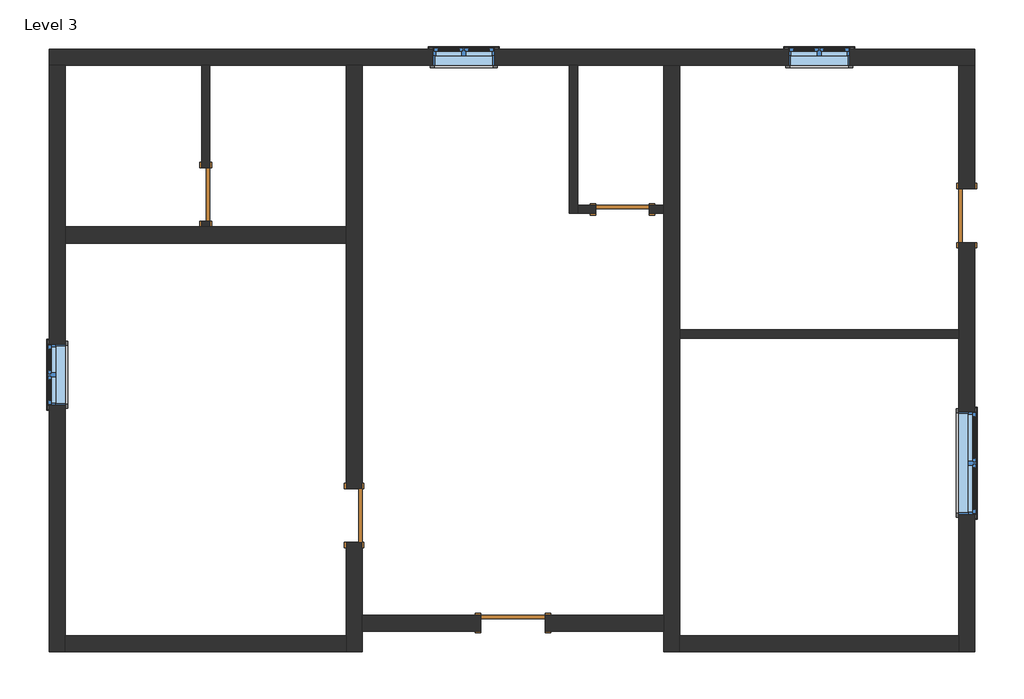
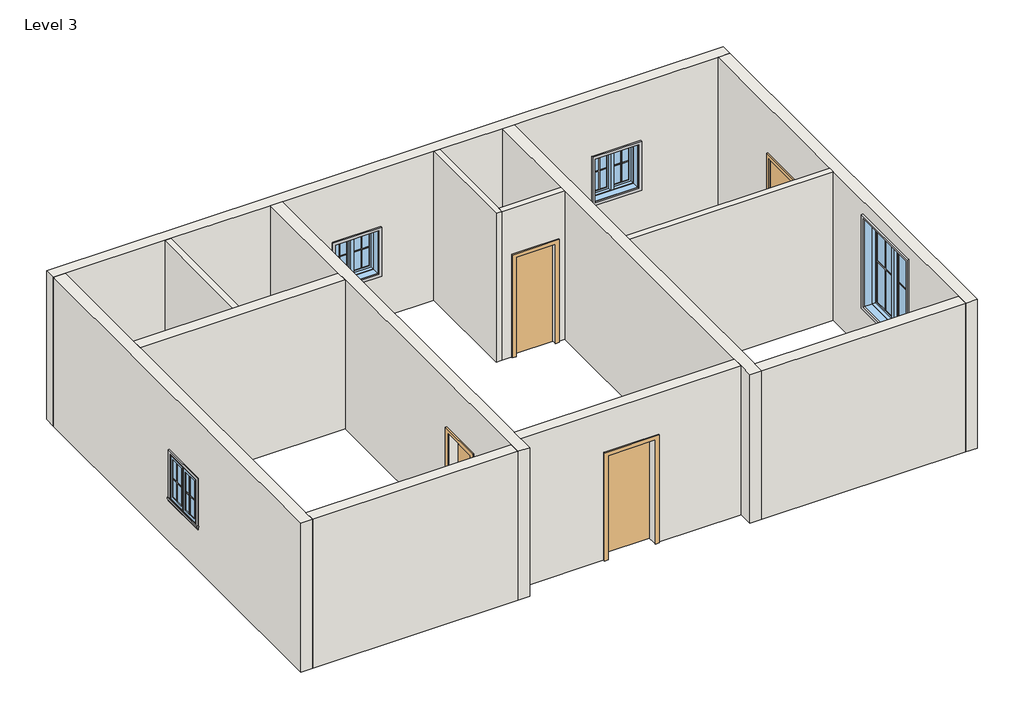
# One storey, incomplete: 16 proxies, 13 walls, 5 doors, 5 windows.
"""IFC4 building model written with IfcOpenShell, lengths in millimetres."""

from ifc_helpers import new_model, si_unit, frame, origin, place, context, project, spatial, polyline, outline, extrude, faceted_brep, transform, mapped, element, save
from components import muntin_pattern_2x2_muntin_pattern_2x2_b3fe6957, muntin_pattern_2x2_muntin_pattern_2x2_3e0ecaf2, muntin_pattern_2x2_muntin_pattern_2x2_bff912c5, muntin_pattern_2x2_muntin_pattern_2x2_c2194282, trim_window_exterior_flat_with_sill_41619996, trim_window_exterior_flat_with_sill_e04b3088, trim_window_interior_flat_picture_frame_51c85655, trim_window_interior_flat_picture_frame_2a7685fe, door_d8f5dbb5, door_f2b275c1, door_85036156, door_0ca8825f, window_aa618e30, window_339605e1, window_9ac97e1a

model = new_model("IFC4")

# Units and contexts
model_context = context("Model", 3, world=origin())
ifc_project = project(units=[si_unit("LENGTHUNIT", "METRE", prefix="MILLI")], contexts=[model_context])

# Site, building, storey
site = spatial("IfcSite", under=ifc_project)
building = spatial("IfcBuilding", under=site)
storey = spatial("IfcBuildingStorey", under=building, Name="Level 3", Elevation=3200.4)

# Proxies
placement = place(None, origin())
muntin_pattern_2x2_muntin_pattern_2x2_shape = muntin_pattern_2x2_muntin_pattern_2x2_b3fe6957(model_context)
element("IfcBuildingElementProxy", 1, Name="Muntin Pattern_2x2 : Muntin Pattern_2x2", ObjectType="Muntin Pattern_2x2 : Muntin Pattern_2x2", at=placement, inside=storey, context=model_context, shape_type="MappedRepresentation", body=[
    mapped(muntin_pattern_2x2_muntin_pattern_2x2_shape, transform((3164.7728376, 7227.4016064, 4184.65), x_axis=(1.0, 0.0, 0.0), y_axis=(0.0, 1.0, 0.0), z_axis=(0.0, 0.0, 1.0))),
])
element("IfcBuildingElementProxy", 2, Name="Muntin Pattern_2x2 : Muntin Pattern_2x2", ObjectType="Muntin Pattern_2x2 : Muntin Pattern_2x2", at=placement, inside=storey, context=model_context, shape_type="MappedRepresentation", body=[
    mapped(muntin_pattern_2x2_muntin_pattern_2x2_shape, transform((-7515.213363, 2411.5985933, 4184.65), x_axis=(0.0, 1.0, 0.0), y_axis=(-1.0, 0.0, 0.0), z_axis=(0.0, 0.0, 1.0))),
])
element("IfcBuildingElementProxy", 3, Name="Muntin Pattern_2x2 : Muntin Pattern_2x2", ObjectType="Muntin Pattern_2x2 : Muntin Pattern_2x2", at=placement, inside=storey, context=model_context, shape_type="MappedRepresentation", body=[
    mapped(muntin_pattern_2x2_muntin_pattern_2x2_shape, transform((-1868.0846872, 7227.4016064, 4184.65), x_axis=(1.0, 0.0, 0.0), y_axis=(0.0, 1.0, 0.0), z_axis=(0.0, 0.0, 1.0))),
])
muntin_pattern_2x2_muntin_pattern_2x2_2_shape = muntin_pattern_2x2_muntin_pattern_2x2_3e0ecaf2(model_context)
element("IfcBuildingElementProxy", 4, Name="Muntin Pattern_2x2 : Muntin Pattern_2x2", ObjectType="Muntin Pattern_2x2 : Muntin Pattern_2x2", at=placement, inside=storey, context=model_context, shape_type="MappedRepresentation", body=[
    mapped(muntin_pattern_2x2_muntin_pattern_2x2_2_shape, transform((3593.3978376, 7227.4016064, 4184.65), x_axis=(-1.0, 0.0, 0.0), y_axis=(0.0, -1.0, 0.0), z_axis=(0.0, 0.0, 1.0))),
])
element("IfcBuildingElementProxy", 5, Name="Muntin Pattern_2x2 : Muntin Pattern_2x2", ObjectType="Muntin Pattern_2x2 : Muntin Pattern_2x2", at=placement, inside=storey, context=model_context, shape_type="MappedRepresentation", body=[
    mapped(muntin_pattern_2x2_muntin_pattern_2x2_2_shape, transform((-7515.213363, 2840.2235933, 4184.65), x_axis=(0.0, -1.0, 0.0), y_axis=(1.0, 0.0, 0.0), z_axis=(0.0, 0.0, 1.0))),
])
element("IfcBuildingElementProxy", 6, Name="Muntin Pattern_2x2 : Muntin Pattern_2x2", ObjectType="Muntin Pattern_2x2 : Muntin Pattern_2x2", at=placement, inside=storey, context=model_context, shape_type="MappedRepresentation", body=[
    mapped(muntin_pattern_2x2_muntin_pattern_2x2_2_shape, transform((-1439.4596872, 7227.4016064, 4184.65), x_axis=(-1.0, 0.0, 0.0), y_axis=(0.0, -1.0, 0.0), z_axis=(0.0, 0.0, 1.0))),
])
muntin_pattern_2x2_muntin_pattern_2x2_3_shape = muntin_pattern_2x2_muntin_pattern_2x2_bff912c5(model_context)
element("IfcBuildingElementProxy", 7, Name="Muntin Pattern_2x2 : Muntin Pattern_2x2", ObjectType="Muntin Pattern_2x2 : Muntin Pattern_2x2", at=placement, inside=storey, context=model_context, shape_type="MappedRepresentation", body=[
    mapped(muntin_pattern_2x2_muntin_pattern_2x2_3_shape, transform((5572.923676, 1735.2928063, 4184.65), x_axis=(0.0, -1.0, 0.0), y_axis=(1.0, 0.0, 0.0), z_axis=(0.0, 0.0, 1.0))),
])
muntin_pattern_2x2_muntin_pattern_2x2_4_shape = muntin_pattern_2x2_muntin_pattern_2x2_c2194282(model_context)
element("IfcBuildingElementProxy", 8, Name="Muntin Pattern_2x2 : Muntin Pattern_2x2", ObjectType="Muntin Pattern_2x2 : Muntin Pattern_2x2", at=placement, inside=storey, context=model_context, shape_type="MappedRepresentation", body=[
    mapped(muntin_pattern_2x2_muntin_pattern_2x2_4_shape, transform((5572.923676, 1014.5678063, 4184.65), x_axis=(0.0, 1.0, 0.0), y_axis=(-1.0, 0.0, 0.0), z_axis=(0.0, 0.0, 1.0))),
])
trim_window_exterior_flat_with_sill_shape = trim_window_exterior_flat_with_sill_41619996(model_context)
element("IfcBuildingElementProxy", 9, Name="Trim-Window-Exterior-Flat : with Sill", ObjectType="Trim-Window-Exterior-Flat : with Sill", at=placement, inside=storey, context=model_context, shape_type="MappedRepresentation", body=[
    mapped(trim_window_exterior_flat_with_sill_shape, transform((3379.0853376, 7236.9266064, 5029.2), x_axis=(-1.0, 0.0, 0.0), y_axis=(0.0, 0.0, 1.0), z_axis=(0.0, 1.0, 0.0))),
])
element("IfcBuildingElementProxy", 10, Name="Trim-Window-Exterior-Flat : with Sill", ObjectType="Trim-Window-Exterior-Flat : with Sill", at=placement, inside=storey, context=model_context, shape_type="MappedRepresentation", body=[
    mapped(trim_window_exterior_flat_with_sill_shape, transform((-7524.738363, 2625.9110933, 5029.2), x_axis=(0.0, -1.0, 0.0), y_axis=(0.0, 0.0, 1.0), z_axis=(-1.0, 0.0, 0.0))),
])
element("IfcBuildingElementProxy", 11, Name="Trim-Window-Exterior-Flat : with Sill", ObjectType="Trim-Window-Exterior-Flat : with Sill", at=placement, inside=storey, context=model_context, shape_type="MappedRepresentation", body=[
    mapped(trim_window_exterior_flat_with_sill_shape, transform((-1653.7721872, 7236.9266064, 5029.2), x_axis=(-1.0, 0.0, 0.0), y_axis=(0.0, 0.0, 1.0), z_axis=(0.0, 1.0, 0.0))),
])
trim_window_exterior_flat_with_sill_2_shape = trim_window_exterior_flat_with_sill_e04b3088(model_context)
element("IfcBuildingElementProxy", 12, Name="Trim-Window-Exterior-Flat : with Sill", ObjectType="Trim-Window-Exterior-Flat : with Sill", at=placement, inside=storey, context=model_context, shape_type="MappedRepresentation", body=[
    mapped(trim_window_exterior_flat_with_sill_2_shape, transform((5582.448676, 1374.9303063, 5943.6), x_axis=(0.0, 1.0, 0.0), y_axis=(0.0, 0.0, 1.0), z_axis=(1.0, 0.0, 0.0))),
])
trim_window_interior_flat_picture_frame_shape = trim_window_interior_flat_picture_frame_51c85655(model_context)
element("IfcBuildingElementProxy", 13, Name="Trim-Window-Interior-Flat : Picture Frame", ObjectType="Trim-Window-Interior-Flat : Picture Frame", at=placement, inside=storey, context=model_context, shape_type="MappedRepresentation", body=[
    mapped(trim_window_interior_flat_picture_frame_shape, transform((3379.0853376, 7008.3266064, 5029.2), x_axis=(1.0, 0.0, 0.0), y_axis=(0.0, 0.0, 1.0), z_axis=(0.0, -1.0, 0.0))),
])
element("IfcBuildingElementProxy", 14, Name="Trim-Window-Interior-Flat : Picture Frame", ObjectType="Trim-Window-Interior-Flat : Picture Frame", at=placement, inside=storey, context=model_context, shape_type="MappedRepresentation", body=[
    mapped(trim_window_interior_flat_picture_frame_shape, transform((-7296.138363, 2625.9110933, 5029.2), x_axis=(0.0, 1.0, 0.0), y_axis=(0.0, 0.0, 1.0), z_axis=(1.0, 0.0, 0.0))),
])
element("IfcBuildingElementProxy", 15, Name="Trim-Window-Interior-Flat : Picture Frame", ObjectType="Trim-Window-Interior-Flat : Picture Frame", at=placement, inside=storey, context=model_context, shape_type="MappedRepresentation", body=[
    mapped(trim_window_interior_flat_picture_frame_shape, transform((-1653.7721872, 7008.3266064, 5029.2), x_axis=(1.0, 0.0, 0.0), y_axis=(0.0, 0.0, 1.0), z_axis=(0.0, -1.0, 0.0))),
])
trim_window_interior_flat_picture_frame_2_shape = trim_window_interior_flat_picture_frame_2a7685fe(model_context)
element("IfcBuildingElementProxy", 16, Name="Trim-Window-Interior-Flat : Picture Frame", ObjectType="Trim-Window-Interior-Flat : Picture Frame", at=placement, inside=storey, context=model_context, shape_type="MappedRepresentation", body=[
    mapped(trim_window_interior_flat_picture_frame_2_shape, transform((5353.848676, 1374.9303063, 5943.6), x_axis=(0.0, -1.0, 0.0), y_axis=(0.0, 0.0, 1.0), z_axis=(-1.0, 0.0, 0.0))),
])

# Doors
door_shape = door_d8f5dbb5(model_context)
element("IfcDoor", 17, ObjectType="Single-Flush : 30\" x 80\"", at=placement, inside=storey, context=model_context, shape_type="MappedRepresentation", body=[
    mapped(door_shape, transform((-5307.8080357, 5179.2254479, 3200.4), x_axis=(0.0, -1.0, 0.0), y_axis=(1.0, 0.0, 0.0), z_axis=(0.0, 0.0, 1.0))),
])
door_2_shape = door_f2b275c1(model_context)
element("IfcDoor", 18, ObjectType="Single-Flush : 30\" x 80\"", at=placement, inside=storey, context=model_context, shape_type="MappedRepresentation", body=[
    mapped(door_2_shape, transform((594.788348, 4969.6493483, 3200.4), x_axis=(-1.0, 0.0, 0.0), y_axis=(0.0, -1.0, 0.0), z_axis=(0.0, 0.0, 1.0))),
])
door_3_shape = door_85036156(model_context)
element("IfcDoor", 19, ObjectType="Single-Flush : 30\" x 80\"", at=placement, inside=storey, context=model_context, shape_type="MappedRepresentation", body=[
    mapped(door_3_shape, transform((5468.148676, 4880.1303063, 3200.4), x_axis=(0.0, -1.0, 0.0), y_axis=(1.0, 0.0, 0.0), z_axis=(0.0, 0.0, 1.0))),
])
element("IfcDoor", 20, ObjectType="Single-Flush : 30\" x 80\"", at=placement, inside=storey, context=model_context, shape_type="MappedRepresentation", body=[
    mapped(door_3_shape, transform((-3207.0990712, 633.8093082, 3200.4), x_axis=(0.0, 1.0, 0.0), y_axis=(-1.0, 0.0, 0.0), z_axis=(0.0, 0.0, 1.0))),
])
door_4_shape = door_0ca8825f(model_context)
element("IfcDoor", 21, ObjectType="Single-Flush : 36\" x 84\"", at=placement, inside=storey, context=model_context, shape_type="MappedRepresentation", body=[
    mapped(door_4_shape, transform((-958.538536, -890.1906918, 3200.4), x_axis=(1.0, 0.0, 0.0), y_axis=(0.0, 1.0, 0.0), z_axis=(0.0, 0.0, 1.0))),
])

# Walls
element("IfcWall", 22, ObjectType="WALL4.5\"", at=placement, inside=storey, context=model_context, shape_type="SweptSolid", body=[
    extrude(outline(polyline([(4798.2254479, 5232.4), (4798.2254479, 3200.4), (4722.0254479, 3200.4), (4722.0254479, 6248.4), (7008.3266064, 6248.4), (7008.3266064, 3200.4), (5560.2254479, 3200.4), (5560.2254479, 5232.4), (4798.2254479, 5232.4)])), frame((-5364.9580357, 0.0, 0.0), z_axis=(1.0, 0.0, 0.0), x_axis=(0.0, 1.0, 0.0)), (0.0, 0.0, 1.0), 114.3),
])
element("IfcWall", 23, ObjectType="WALL4.5\"", at=placement, inside=storey, context=model_context, shape_type="Brep", body=[
    faceted_brep([(-157.5953031, 7008.3266064, 3200.4), (-157.5953031, 4912.4993483, 3200.4), (-157.5953031, 4912.4993483, 6248.4), (-157.5953031, 7008.3266064, 6248.4), (-43.2953031, 7008.3266064, 3200.4), (-43.2953031, 7008.3266064, 6248.4), (-43.2953031, 5026.7993483, 6248.4), (-43.2953031, 4912.4993483, 6248.4), (-43.2953031, 4912.4993483, 3200.4), (-43.2953031, 5026.7993483, 3200.4)], [[[0, 1, 2, 3]], [[4, 5, 6, 7, 8, 9]], [[1, 0, 4, 9, 8]], [[0, 3, 5, 4]], [[2, 1, 8, 7]], [[3, 2, 7, 6, 5]]]),
])
element("IfcWall", 24, ObjectType="WALL4.5\"", at=placement, inside=storey, context=model_context, shape_type="SweptSolid", body=[
    extrude(outline(polyline([(3200.4, -43.2953031), (3200.4, 213.788348), (5232.4, 213.788348), (5232.4, 975.788348), (3200.4, 975.788348), (3200.4, 1175.7219991), (6248.4, 1175.7219991), (6248.4, -43.2953031), (3200.4, -43.2953031)])), frame((0.0, 4912.4993483, 0.0), z_axis=(0.0, 1.0, 0.0), x_axis=(0.0, 0.0, 1.0)), (0.0, 0.0, 1.0), 114.3),
])
element("IfcWall", 25, ObjectType="WALL4.5\"", at=placement, inside=storey, context=model_context, shape_type="SweptSolid", body=[
    extrude(outline(polyline([(1404.3219991, 3260.8803063), (5353.848676, 3260.8803063), (5353.848676, 3146.5803063), (1404.3219991, 3146.5803063), (1404.3219991, 3260.8803063)])), frame((0.0, 0.0, 3200.4), z_axis=(0.0, 0.0, 1.0), x_axis=(1.0, 0.0, 0.0)), (0.0, 0.0, 1.0), 3048.0),
])
element("IfcWall", 26, ObjectType="WALL9\"", at=placement, inside=storey, context=model_context, shape_type="Brep", body=[
    faceted_brep([(-7524.738363, 7008.3266064, 3200.4), (-7296.138363, 7008.3266064, 3200.4), (-5364.9580357, 7008.3266064, 3200.4), (-5250.6580357, 7008.3266064, 3200.4), (-3321.3990712, 7008.3266064, 3200.4), (-3092.7990712, 7008.3266064, 3200.4), (-157.5953031, 7008.3266064, 3200.4), (-43.2953031, 7008.3266064, 3200.4), (1175.7219991, 7008.3266064, 3200.4), (1404.3219991, 7008.3266064, 3200.4), (5353.848676, 7008.3266064, 3200.4), (5582.448676, 7008.3266064, 3200.4), (5582.448676, 7008.3266064, 6248.4), (5353.848676, 7008.3266064, 6248.4), (1404.3219991, 7008.3266064, 6248.4), (1175.7219991, 7008.3266064, 6248.4), (-43.2953031, 7008.3266064, 6248.4), (-157.5953031, 7008.3266064, 6248.4), (-3092.7990712, 7008.3266064, 6248.4), (-3321.3990712, 7008.3266064, 6248.4), (-5250.6580357, 7008.3266064, 6248.4), (-5364.9580357, 7008.3266064, 6248.4), (-7296.138363, 7008.3266064, 6248.4), (-7524.738363, 7008.3266064, 6248.4), (-4054.2535534, 7008.3266064, 3987.8), (-4054.2535534, 7008.3266064, 3378.2), (-4460.6535534, 7008.3266064, 3378.2), (-4460.6535534, 7008.3266064, 3987.8), (3810.8853376, 7008.3266064, 5029.2), (3810.8853376, 7008.3266064, 4114.8), (2947.2853376, 7008.3266064, 4114.8), (2947.2853376, 7008.3266064, 5029.2), (-1221.9721872, 7008.3266064, 5029.2), (-1221.9721872, 7008.3266064, 4114.8), (-2085.5721872, 7008.3266064, 4114.8), (-2085.5721872, 7008.3266064, 5029.2), (-7524.738363, 7236.9266064, 3200.4), (-7524.738363, 7236.9266064, 6248.4), (5582.448676, 7236.9266064, 6248.4), (5582.448676, 7236.9266064, 3200.4), (-4054.2535534, 7236.9266064, 3987.8), (-4460.6535534, 7236.9266064, 3987.8), (-4460.6535534, 7236.9266064, 3378.2), (-4054.2535534, 7236.9266064, 3378.2), (3810.8853376, 7236.9266064, 5029.2), (2947.2853376, 7236.9266064, 5029.2), (2947.2853376, 7236.9266064, 4114.8), (3810.8853376, 7236.9266064, 4114.8), (-1221.9721872, 7236.9266064, 5029.2), (-2085.5721872, 7236.9266064, 5029.2), (-2085.5721872, 7236.9266064, 4114.8), (-1221.9721872, 7236.9266064, 4114.8)], [[[0, 1, 2, 3, 4, 5, 6, 7, 8, 9, 10, 11, 12, 13, 14, 15, 16, 17, 18, 19, 20, 21, 22, 23], [24, 25, 26, 27], [28, 29, 30, 31], [32, 33, 34, 35]], [[36, 37, 38, 39], [40, 41, 42, 43], [44, 45, 46, 47], [48, 49, 50, 51]], [[11, 10, 9, 8, 7, 6, 5, 4, 3, 2, 1, 0, 36, 39]], [[12, 11, 39, 38]], [[0, 23, 37, 36]], [[23, 22, 21, 20, 19, 18, 17, 16, 15, 14, 13, 12, 38, 37]], [[25, 24, 40, 43]], [[26, 25, 43, 42]], [[27, 26, 42, 41]], [[24, 27, 41, 40]], [[29, 28, 44, 47]], [[30, 29, 47, 46]], [[31, 30, 46, 45]], [[28, 31, 45, 44]], [[33, 32, 48, 51]], [[34, 33, 51, 50]], [[35, 34, 50, 49]], [[32, 35, 49, 48]]]),
])
element("IfcWall", 27, ObjectType="WALL9\"", at=placement, inside=storey, context=model_context, shape_type="Brep", body=[
    faceted_brep([(5353.848676, 4499.1303063, 5232.4), (5353.848676, 4499.1303063, 3200.4), (5353.848676, 3260.8803063, 3200.4), (5353.848676, 3146.5803063, 3200.4), (5353.848676, -1070.2868249, 3200.4), (5353.848676, -1298.8868249, 3200.4), (5353.848676, -1298.8868249, 6248.4), (5353.848676, -1070.2868249, 6248.4), (5353.848676, 3146.5803063, 6248.4), (5353.848676, 3260.8803063, 6248.4), (5353.848676, 7008.3266064, 6248.4), (5353.848676, 7008.3266064, 3200.4), (5353.848676, 5261.1303063, 3200.4), (5353.848676, 5261.1303063, 5232.4), (5353.848676, 651.0303063, 5943.6), (5353.848676, 651.0303063, 4114.8), (5353.848676, 2098.8303063, 4114.8), (5353.848676, 2098.8303063, 5943.6), (5582.448676, -1298.8868249, 3200.4), (5582.448676, 4499.1303063, 3200.4), (5582.448676, 4499.1303063, 5232.4), (5582.448676, 5261.1303063, 5232.4), (5582.448676, 5261.1303063, 3200.4), (5582.448676, 7008.3266064, 3200.4), (5582.448676, 7008.3266064, 6248.4), (5582.448676, -1298.8868249, 6248.4), (5582.448676, 651.0303063, 5943.6), (5582.448676, 2098.8303063, 5943.6), (5582.448676, 2098.8303063, 4114.8), (5582.448676, 651.0303063, 4114.8)], [[[0, 1, 2, 3, 4, 5, 6, 7, 8, 9, 10, 11, 12, 13], [14, 15, 16, 17]], [[18, 19, 20, 21, 22, 23, 24, 25], [26, 27, 28, 29]], [[12, 11, 23, 22]], [[5, 4, 3, 2, 1, 19, 18]], [[11, 10, 24, 23]], [[6, 5, 18, 25]], [[20, 19, 1, 0]], [[21, 20, 0, 13]], [[22, 21, 13, 12]], [[10, 9, 8, 7, 6, 25, 24]], [[15, 14, 26, 29]], [[16, 15, 29, 28]], [[17, 16, 28, 27]], [[14, 17, 27, 26]]]),
])
element("IfcWall", 28, ObjectType="WALL9\"", at=placement, inside=storey, context=model_context, shape_type="Brep", body=[
    faceted_brep([(-7296.138363, -1298.8868249, 3200.4), (-7296.138363, -1070.2868249, 3200.4), (-7296.138363, 4492.8110933, 3200.4), (-7296.138363, 4721.4110933, 3200.4), (-7296.138363, 7008.3266064, 3200.4), (-7296.138363, 7008.3266064, 6248.4), (-7296.138363, 4721.4110933, 6248.4), (-7296.138363, 4492.8110933, 6248.4), (-7296.138363, -1070.2868249, 6248.4), (-7296.138363, -1298.8868249, 6248.4), (-7296.138363, 3057.7110933, 5029.2), (-7296.138363, 3057.7110933, 4114.8), (-7296.138363, 2194.1110933, 4114.8), (-7296.138363, 2194.1110933, 5029.2), (-7524.738363, -1298.8868249, 3200.4), (-7524.738363, -1298.8868249, 6248.4), (-7524.738363, 7008.3266064, 6248.4), (-7524.738363, 7008.3266064, 3200.4), (-7524.738363, 3057.7110933, 5029.2), (-7524.738363, 2194.1110933, 5029.2), (-7524.738363, 2194.1110933, 4114.8), (-7524.738363, 3057.7110933, 4114.8)], [[[0, 1, 2, 3, 4, 5, 6, 7, 8, 9], [10, 11, 12, 13]], [[14, 15, 16, 17], [18, 19, 20, 21]], [[4, 3, 2, 1, 0, 14, 17]], [[5, 4, 17, 16]], [[0, 9, 15, 14]], [[9, 8, 7, 6, 5, 16, 15]], [[11, 10, 18, 21]], [[12, 11, 21, 20]], [[13, 12, 20, 19]], [[10, 13, 19, 18]]]),
])
element("IfcWall", 29, ObjectType="WALL9\"", at=placement, inside=storey, context=model_context, shape_type="Brep", body=[
    faceted_brep([(-3321.3990712, 7008.3266064, 3200.4), (-3321.3990712, 4721.4110933, 3200.4), (-3321.3990712, 4492.8110933, 3200.4), (-3321.3990712, 1014.8093082, 3200.4), (-3321.3990712, 1014.8093082, 5232.4), (-3321.3990712, 252.8093082, 5232.4), (-3321.3990712, 252.8093082, 3200.4), (-3321.3990712, -1070.2868249, 3200.4), (-3321.3990712, -1298.8868249, 3200.4), (-3321.3990712, -1298.8868249, 6248.4), (-3321.3990712, -1070.2868249, 6248.4), (-3321.3990712, 4492.8110933, 6248.4), (-3321.3990712, 4721.4110933, 6248.4), (-3321.3990712, 7008.3266064, 6248.4), (-3092.7990712, 1014.8093082, 5232.4), (-3092.7990712, 1014.8093082, 3200.4), (-3092.7990712, 7008.3266064, 3200.4), (-3092.7990712, 7008.3266064, 6248.4), (-3092.7990712, -775.8906918, 6248.4), (-3092.7990712, -1004.4906918, 6248.4), (-3092.7990712, -1298.8868249, 6248.4), (-3092.7990712, -1298.8868249, 3200.4), (-3092.7990712, -1004.4906918, 3200.4), (-3092.7990712, -775.8906918, 3200.4), (-3092.7990712, 252.8093082, 3200.4), (-3092.7990712, 252.8093082, 5232.4)], [[[0, 1, 2, 3, 4, 5, 6, 7, 8, 9, 10, 11, 12, 13]], [[14, 15, 16, 17, 18, 19, 20, 21, 22, 23, 24, 25]], [[16, 15, 3, 2, 1, 0]], [[24, 23, 22, 21, 8, 7, 6]], [[0, 13, 17, 16]], [[9, 8, 21, 20]], [[4, 3, 15, 14]], [[5, 4, 14, 25]], [[6, 5, 25, 24]], [[13, 12, 11, 10, 9, 20, 19, 18, 17]]]),
])
element("IfcWall", 30, ObjectType="WALL9\"", at=placement, inside=storey, context=model_context, shape_type="Brep", body=[
    faceted_brep([(1175.7219991, 7008.3266064, 3200.4), (1175.7219991, 5026.7993483, 3200.4), (1175.7219991, 4912.4993483, 3200.4), (1175.7219991, -775.8906918, 3200.4), (1175.7219991, -1004.4906918, 3200.4), (1175.7219991, -1298.8868249, 3200.4), (1175.7219991, -1298.8868249, 6248.4), (1175.7219991, -1004.4906918, 6248.4), (1175.7219991, -775.8906918, 6248.4), (1175.7219991, 4912.4993483, 6248.4), (1175.7219991, 5026.7993483, 6248.4), (1175.7219991, 7008.3266064, 6248.4), (1404.3219991, 7008.3266064, 3200.4), (1404.3219991, 7008.3266064, 6248.4), (1404.3219991, 3260.8803063, 6248.4), (1404.3219991, 3146.5803063, 6248.4), (1404.3219991, -1070.2868249, 6248.4), (1404.3219991, -1298.8868249, 6248.4), (1404.3219991, -1298.8868249, 3200.4), (1404.3219991, -1070.2868249, 3200.4), (1404.3219991, 3146.5803063, 3200.4), (1404.3219991, 3260.8803063, 3200.4)], [[[0, 1, 2, 3, 4, 5, 6, 7, 8, 9, 10, 11]], [[12, 13, 14, 15, 16, 17, 18, 19, 20, 21]], [[5, 4, 3, 2, 1, 0, 12, 21, 20, 19, 18]], [[0, 11, 13, 12]], [[6, 5, 18, 17]], [[11, 10, 9, 8, 7, 6, 17, 16, 15, 14, 13]]]),
])
element("IfcWall", 31, ObjectType="WALL9\"", at=placement, inside=storey, context=model_context, shape_type="SweptSolid", body=[
    extrude(outline(polyline([(-3321.3990712, -1298.8868249), (-7296.138363, -1298.8868249), (-7296.138363, -1070.2868249), (-3321.3990712, -1070.2868249), (-3321.3990712, -1298.8868249)])), frame((0.0, 0.0, 3200.4), z_axis=(0.0, 0.0, 1.0), x_axis=(1.0, 0.0, 0.0)), (0.0, 0.0, 1.0), 3048.0),
])
element("IfcWall", 32, ObjectType="WALL9\"", at=placement, inside=storey, context=model_context, shape_type="SweptSolid", body=[
    extrude(outline(polyline([(5353.848676, -1298.8868249), (1404.3219991, -1298.8868249), (1404.3219991, -1070.2868249), (5353.848676, -1070.2868249), (5353.848676, -1298.8868249)])), frame((0.0, 0.0, 3200.4), z_axis=(0.0, 0.0, 1.0), x_axis=(1.0, 0.0, 0.0)), (0.0, 0.0, 1.0), 3048.0),
])
element("IfcWall", 33, ObjectType="WALL9\"", at=placement, inside=storey, context=model_context, shape_type="SweptSolid", body=[
    extrude(outline(polyline([(5334.0, -501.338536), (3200.4, -501.338536), (3200.4, 1175.7219991), (6248.4, 1175.7219991), (6248.4, -3092.7990712), (3200.4, -3092.7990712), (3200.4, -1415.738536), (5334.0, -1415.738536), (5334.0, -501.338536)])), frame((0.0, -1004.4906918, 0.0), z_axis=(0.0, 1.0, 0.0), x_axis=(0.0, 0.0, 1.0)), (0.0, 0.0, 1.0), 228.6),
])
element("IfcWall", 34, ObjectType="WALL9\"", at=placement, inside=storey, context=model_context, shape_type="SweptSolid", body=[
    extrude(outline(polyline([(-3321.3990712, 4492.8110933), (-7296.138363, 4492.8110933), (-7296.138363, 4721.4110933), (-3321.3990712, 4721.4110933), (-3321.3990712, 4492.8110933)])), frame((0.0, 0.0, 3200.4), z_axis=(0.0, 0.0, 1.0), x_axis=(1.0, 0.0, 0.0)), (0.0, 0.0, 1.0), 3048.0),
])

# Windows
window_shape = window_aa618e30(model_context)
element("IfcWindow", 35, ObjectType="Fixed : 16\" x 24\"", at=placement, inside=storey, context=model_context, shape_type="MappedRepresentation", body=[
    mapped(window_shape, transform((-4219.3535534, 7122.6266064, 2463.8), x_axis=(1.0, 0.0, 0.0), y_axis=(0.0, 1.0, 0.0), z_axis=(0.0, 0.0, 1.0))),
])
window_2_shape = window_339605e1(model_context)
element("IfcWindow", 36, ObjectType="Window-Casement-Double : 34\" x 36\"", at=placement, inside=storey, context=model_context, shape_type="MappedRepresentation", body=[
    mapped(window_2_shape, transform((3379.0853376, 7122.6266064, 3200.4), x_axis=(1.0, 0.0, 0.0), y_axis=(0.0, 1.0, 0.0), z_axis=(0.0, 0.0, 1.0))),
])
element("IfcWindow", 37, ObjectType="Window-Casement-Double : 34\" x 36\"", at=placement, inside=storey, context=model_context, shape_type="MappedRepresentation", body=[
    mapped(window_2_shape, transform((-7410.438363, 2625.9110933, 3200.4), x_axis=(0.0, 1.0, 0.0), y_axis=(-1.0, 0.0, 0.0), z_axis=(0.0, 0.0, 1.0))),
])
element("IfcWindow", 38, ObjectType="Window-Casement-Double : 34\" x 36\"", at=placement, inside=storey, context=model_context, shape_type="MappedRepresentation", body=[
    mapped(window_2_shape, transform((-1653.7721872, 7122.6266064, 3200.4), x_axis=(1.0, 0.0, 0.0), y_axis=(0.0, 1.0, 0.0), z_axis=(0.0, 0.0, 1.0))),
])
window_3_shape = window_9ac97e1a(model_context)
element("IfcWindow", 39, ObjectType="Window-Casement-Double : 57\" x 72\"", at=placement, inside=storey, context=model_context, shape_type="MappedRepresentation", body=[
    mapped(window_3_shape, transform((5468.148676, 1374.9303063, 3200.4), x_axis=(0.0, -1.0, 0.0), y_axis=(1.0, 0.0, 0.0), z_axis=(0.0, 0.0, 1.0))),
])

save(model, "model.ifc")

# Revit data of these elements
# Type "Muntin Pattern_2x2 : Muntin Pattern_2x2"
#   Width [instance default] = 4' - 0"
#   Thickness = 0' - 0 1/2"
#   Height [instance default] = 4' - 0"
#   Distance = 0' - 0 3/4"
#   Interior Material [instance default] = none
#   Exterior Material [instance default] = none
#   Default Elevation = 0
# Type "Trim-Window-Exterior-Flat : with Sill"
#   Trim Width = 0' - 2 1/4"
#   Trim Thickness_Picture Frame = 0' - 1 1/4"
#   Trim Thickness_with Sill = 0' - 0 3/4"
#   Sill Thickness = 0' - 1 1/4"
#   Opening Width [instance default] = 2' - 0"
#   Opening Height [instance default] = 3' - 0"
#   Default Elevation = 4' - 0"
#   Sill = yes
#   Picture Frame = no
#   Trim Material [instance default] = none
# Type "Trim-Window-Interior-Flat : Picture Frame"
#   Trim Thickness_Picture Frame = 0' - 1 1/4"
#   Trim Width = 0' - 2 1/4"
#   Trim Thickness_with Sill = 0' - 0 3/4"
#   Sill Thickness = 0' - 1 1/4"
#   Opening Width [instance default] = 2' - 0"
#   Opening Height [instance default] = 3' - 0"
#   Default Elevation = 4' - 0"
#   Sill = no
#   Picture Frame = yes
#   Trim Material [instance default] = none
# Type "Single-Flush : 30\" x 80\""
#   Type Mark = "5"
#   Construction Type Id = "MDOOR"
#   Assembly Code = "C1020"
#   Analytic Construction = "Metal"
#   Thickness = 0' - 2"
#   Heat Transfer Coefficient (U) = 0.651978 BTU/(h·ft²·°F)
#   Height = 6' - 8"
#   Trim Projection Ext = 0' - 1"
#   Trim Projection Int = 0' - 1"
#   Trim Width = 0' - 3"
#   Width = 2' - 6"
#   Define Thermal Properties by = 1
#   Define Thermal Properties by = 1
#   Door Material = Door - Panel
#   Frame Material = Door - Frame
#   Visual Light Transmittance = 0
#   Solar Heat Gain Coefficient = 0
#   Function = (empty or 0)
#   Wall Closure = (empty or 0)
# Type "Single-Flush : 36\" x 84\""
#   Type Mark = "1"
#   Construction Type Id = "MDOOR"
#   Assembly Code = "C1020"
#   Analytic Construction = "Metal"
#   Thickness = 0' - 2"
#   Heat Transfer Coefficient (U) = 0.651978 BTU/(h·ft²·°F)
#   Height = 7' - 0"
#   Trim Projection Ext = 0' - 1"
#   Trim Projection Int = 0' - 1"
#   Trim Width = 0' - 3"
#   Width = 3' - 0"
#   Define Thermal Properties by = 1
#   Define Thermal Properties by = 1
#   Door Material = Door - Panel
#   Frame Material = Door - Frame
#   Visual Light Transmittance = 0
#   Solar Heat Gain Coefficient = 0
#   Function = (empty or 0)
#   Wall Closure = (empty or 0)
# Type "WALL4.5\""
#   Assembly Code = "B2010"
#   Layers, outside or top first: 0' - 4 1/2" no material (function 1)
# Type "WALL9\""
#   Assembly Code = "B2010"
#   Layers, outside or top first: 0' - 9" no material (function 1)
# Type "Fixed : 16\" x 24\""
#   Type Mark = "4"
#   Construction Type Id = "GSP4R"
#   Assembly Code = "B2020100"
#   Analytic Construction = "1/8 in Pilkington single glazing"
#   Visual Light Transmittance = 0.9
#   Solar Heat Gain Coefficient = 0.78
#   Heat Transfer Coefficient (U) = 0.6496 BTU/(h·ft²·°F)
#   Height = 2' - 0"
#   Default Sill Height = 3' - 0"
#   Width = 1' - 4"
#   Window Inset = 0' - 0 3/4"
#   Define Thermal Properties by = 1
#   Define Thermal Properties by = 1
#   Glass Pane Material = Glass
#   Sash Material = Sash
#   Wall Closure = (empty or 0)
# Type "Window-Casement-Double : 34\" x 36\""
#   Type Mark = "14"
#   Fire Rating = "0.5h"
#   Assembly Code = "B2020100"
#   Analytic Construction = "Double glazing - domestic"
#   Frame Extension [instance default] = 0' - 0 1/4"
#   Window Inset [instance default] = 0' - 0"
#   Wall Thickness [instance default] = 0' - 6"
#   Interior Wall Closure [instance default] = 0' - 2 1/4"
#   Half Width = 1' - 5"
#   Visual Light Transmittance = 0.81
#   Thermal Resistance (R) = 1.8146 (h·ft²·°F)/BTU
#   Solar Heat Gain Coefficient = 0.76
#   Rough Width = 2' - 10 1/2"
#   Rough Height = 3' - 0 1/2"
#   Height = 3' - 0"
#   Heat Transfer Coefficient (U) = 0.5511 BTU/(h·ft²·°F)
#   Exterior Wall Closure [instance default] = 0' - 1 1/4"
#   Extension Jamb [instance default] = 0' - 2 1/4"
#   Default Sill Height = 3' - 0"
#   Width = 2' - 10"
#   Define Thermal Properties by = 0
#   Muntin Visibility = yes
#   Interior Trim Visibility [instance default] = yes
#   Exterior Trim Visibility [instance default] = yes
#   Extension Jamb Visibility [instance default] = yes
#   Interior Trim Material = Wood - Stained
#   Muntin Pattern = Muntin Pattern_2x2 : Muntin Pattern_2x2
#   Interior Trim = Trim-Window-Interior-Flat : Picture Frame
#   Interior Frame Material = Wood - Stained
#   Glass Panel Material = Glass
#   Exterior Trim Material = Clad - White
#   Exterior Trim = Trim-Window-Exterior-Flat : with Sill
#   Exterior Frame Material = Clad - White
#   Wall Closure = (empty or 0)
# Type "Window-Casement-Double : 57\" x 72\""
#   Type Mark = "17"
#   Fire Rating = "0.5h"
#   Assembly Code = "B2020100"
#   Analytic Construction = "Double glazing - domestic"
#   Frame Extension [instance default] = 0' - 0 1/4"
#   Window Inset [instance default] = 0' - 0"
#   Wall Thickness [instance default] = 0' - 6"
#   Interior Wall Closure [instance default] = 0' - 2 1/4"
#   Half Width = 2' - 4 1/2"
#   Visual Light Transmittance = 0.81
#   Thermal Resistance (R) = 1.8146 (h·ft²·°F)/BTU
#   Solar Heat Gain Coefficient = 0.76
#   Rough Width = 4' - 9 1/2"
#   Rough Height = 6' - 0 1/2"
#   Height = 6' - 0"
#   Heat Transfer Coefficient (U) = 0.5511 BTU/(h·ft²·°F)
#   Exterior Wall Closure [instance default] = 0' - 1 1/4"
#   Extension Jamb [instance default] = 0' - 2 1/4"
#   Default Sill Height = 3' - 0"
#   Width = 4' - 9"
#   Define Thermal Properties by = 0
#   Muntin Visibility = yes
#   Interior Trim Visibility [instance default] = yes
#   Exterior Trim Visibility [instance default] = yes
#   Extension Jamb Visibility [instance default] = yes
#   Interior Trim Material = Wood - Stained
#   Muntin Pattern = Muntin Pattern_2x2 : Muntin Pattern_2x2
#   Interior Trim = Trim-Window-Interior-Flat : Picture Frame
#   Interior Frame Material = Wood - Stained
#   Glass Panel Material = Glass
#   Exterior Trim Material = Clad - White
#   Exterior Trim = Trim-Window-Exterior-Flat : with Sill
#   Exterior Frame Material = Clad - White
#   Wall Closure = (empty or 0)
# Elements 1, 2, 3, 4, 5, 6 (IfcBuildingElementProxy, "Muntin Pattern_2x2 : Muntin Pattern_2x2")
#   Width = 0' - 11 5/8"
#   Height = 2' - 6 1/2"
#   Interior Material = Wood - Stained
#   Exterior Material = Clad - White
#   Phase Created = New Construction
#   Materials on its faces: "Clad - White", "Wood - Stained"
# Elements 7, 8 (IfcBuildingElementProxy, "Muntin Pattern_2x2 : Muntin Pattern_2x2")
#   Width = 1' - 11 1/8"
#   Height = 5' - 6 1/2"
#   Interior Material = Wood - Stained
#   Exterior Material = Clad - White
#   Phase Created = New Construction
#   Materials on its faces: "Clad - White", "Wood - Stained"
# Elements 9, 10, 11 (IfcBuildingElementProxy, "Trim-Window-Exterior-Flat : with Sill")
#   Opening Width = 2' - 10"
#   Opening Height = 3' - 0"
#   Trim Material = Clad - White
#   Phase Created = New Construction
#   Materials on its faces: "Clad - White"
# Element 12 (IfcBuildingElementProxy, "Trim-Window-Exterior-Flat : with Sill")
#   Opening Width = 4' - 9"
#   Opening Height = 6' - 0"
#   Trim Material = Clad - White
#   Phase Created = New Construction
#   Materials on its faces: "Clad - White"
# Elements 13, 14, 15 (IfcBuildingElementProxy, "Trim-Window-Interior-Flat : Picture Frame")
#   Opening Width = 2' - 10"
#   Opening Height = 3' - 0"
#   Trim Material = Wood - Stained
#   Phase Created = New Construction
#   Materials on its faces: "Wood - Stained"
# Element 16 (IfcBuildingElementProxy, "Trim-Window-Interior-Flat : Picture Frame")
#   Opening Width = 4' - 9"
#   Opening Height = 6' - 0"
#   Trim Material = Wood - Stained
#   Phase Created = New Construction
#   Materials on its faces: "Wood - Stained"
# Elements 17, 18, 19, 20 (IfcDoor, "Single-Flush : 30\" x 80\"")
#   Phase Created = New Construction
#   Materials on its faces: "Door - Frame", "Door - Panel"
# Element 21 (IfcDoor, "Single-Flush : 36\" x 84\"")
#   Phase Created = New Construction
#   Materials on its faces: "Door - Frame", "Door - Panel"
# Elements 22, 23, 24, 25 (IfcWall, "WALL4.5\"")
#   Top Offset = 0' - 0"
#   Base Offset = 0' - 0"
#   Unconnected Height = 10' - 0"
#   wall height = 10' - 0"
#   Phase Created = New Construction
#   Base Constraint = Level 3
#   Materials on its faces: "Default Wall"
# Elements 26, 27, 28, 29, 30, 31, 32, 33 (IfcWall, "WALL9\"")
#   Top Offset = 0' - 0"
#   Base Offset = 0' - 0"
#   Unconnected Height = 10' - 0"
#   wall height = 10' - 0"
#   Phase Created = New Construction
#   Base Constraint = Level 3
#   Materials on its faces: "Default Wall", "Blanket"
# Element 34 (IfcWall, "WALL9\"")
#   Top Offset = 0' - 0"
#   Base Offset = 0' - 0"
#   Unconnected Height = 10' - 0"
#   wall height = 10' - 0"
#   Phase Created = New Construction
#   Base Constraint = Level 3
#   Materials on its faces: "Default Wall"
# Element 35 (IfcWindow, "Fixed : 16\" x 24\"")
#   Mark = "6"
#   Phase Created = New Construction
#   Materials on its faces: "Sash", "Glass"
# Element 36 (IfcWindow, "Window-Casement-Double : 34\" x 36\"")
#   Mark = "7"
#   Window Inset = 0' - 0"
#   Interior Wall Closure = 0' - 2 1/4"
#   Frame Extension = 0' - 0 1/4"
#   Exterior Wall Closure = 0' - 1 1/4"
#   Interior Trim Visibility = yes
#   Exterior Trim Visibility = yes
#   Phase Created = New Construction
#   Materials on its faces: "Wood - Stained", "Glass", "Clad - White"
# Element 37 (IfcWindow, "Window-Casement-Double : 34\" x 36\"")
#   Mark = "8"
#   Window Inset = 0' - 0"
#   Interior Wall Closure = 0' - 2 1/4"
#   Frame Extension = 0' - 0 1/4"
#   Exterior Wall Closure = 0' - 1 1/4"
#   Interior Trim Visibility = yes
#   Exterior Trim Visibility = yes
#   Phase Created = New Construction
#   Materials on its faces: "Wood - Stained", "Glass", "Clad - White"
# Element 38 (IfcWindow, "Window-Casement-Double : 34\" x 36\"")
#   Mark = "10"
#   Window Inset = 0' - 0"
#   Interior Wall Closure = 0' - 2 1/4"
#   Frame Extension = 0' - 0 1/4"
#   Exterior Wall Closure = 0' - 1 1/4"
#   Interior Trim Visibility = yes
#   Exterior Trim Visibility = yes
#   Phase Created = New Construction
#   Materials on its faces: "Wood - Stained", "Glass", "Clad - White"
# Element 39 (IfcWindow, "Window-Casement-Double : 57\" x 72\"")
#   Mark = "9"
#   Window Inset = 0' - 0"
#   Interior Wall Closure = 0' - 2 1/4"
#   Frame Extension = 0' - 0 1/4"
#   Exterior Wall Closure = 0' - 1 1/4"
#   Interior Trim Visibility = yes
#   Exterior Trim Visibility = yes
#   Phase Created = New Construction
#   Materials on its faces: "Wood - Stained", "Glass", "Clad - White"
# Materials
#   "Door - Panel": class "Wood", colour RGB 210 159 95, transparency 0, Cost = 0
#   "Door - Frame": colour RGB 118 70 51, transparency 0, Cost = 0
#   "Glass": class "Glass", colour RGB 0 128 192, transparency 0.75, Description = "Soda Lime Glass", Cost = 0
#   "Sash": class "Wood", colour RGB 224 178 126, transparency 0, Cost = 0
#   "Wood - Stained": class "Wood", colour RGB 224 178 126, transparency 0, Cost = 0
#   "Clad - White": class "Wood", colour RGB 242 242 238, transparency 0, Cost = 0
#   "Default Wall": colour RGB 128 128 128, transparency 0, Cost = 0
#   "Blanket": class "System", colour RGB 59 0 1, transparency 0, Cost = 0
